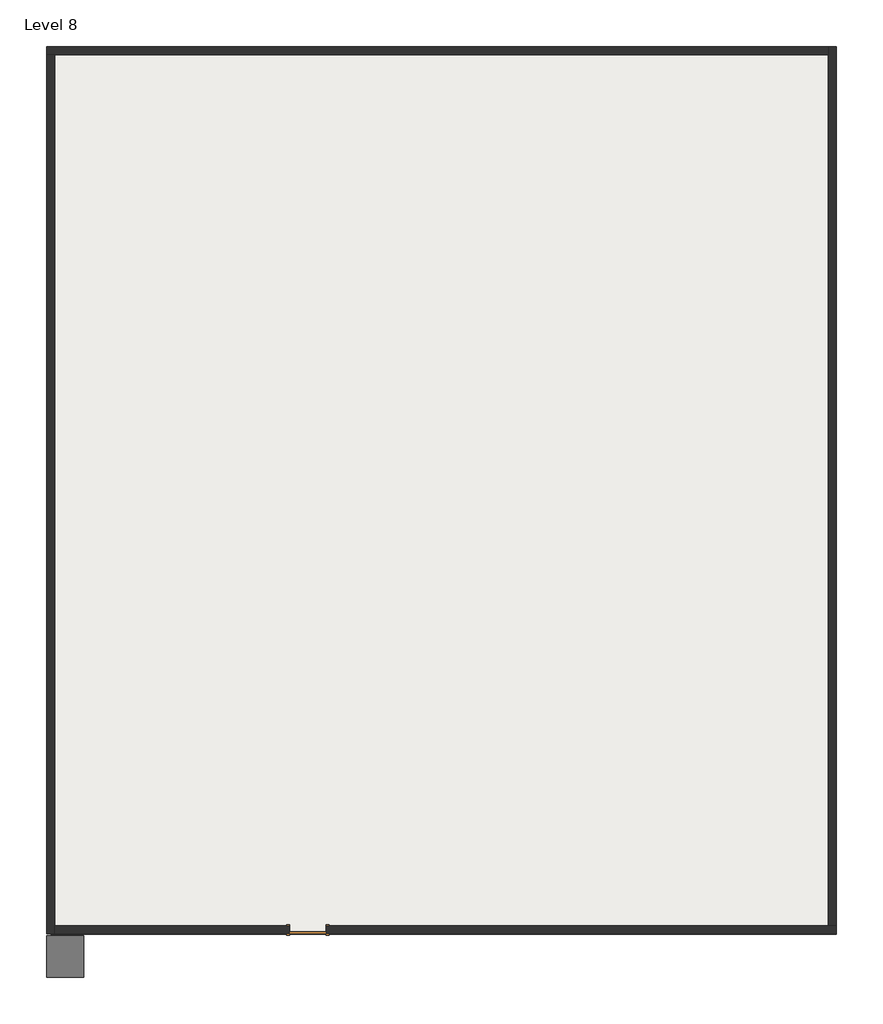
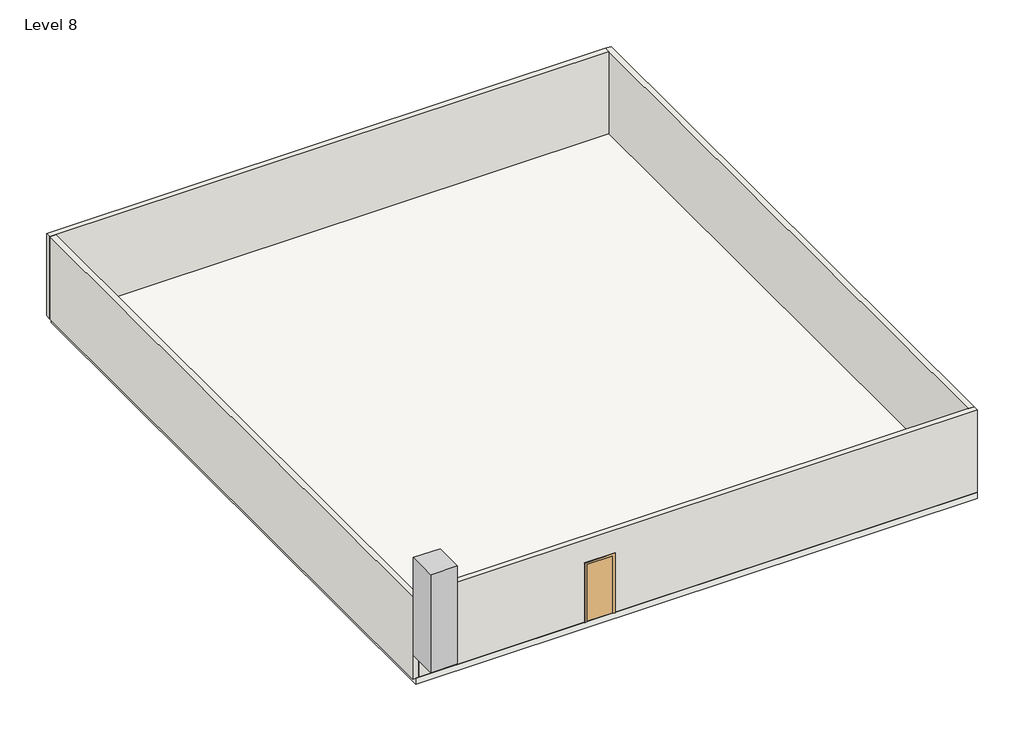
# One storey: 4 walls, 1 door, 1 proxy, 1 roof.
"""IFC4 building model written with IfcOpenShell, lengths in millimetres."""

from ifc_helpers import new_model, si_unit, frame, origin, place, context, project, spatial, polyline, outline, extrude, faceted_brep, transform, mapped, element, save
from components import generic_models_4_generic_models_4_47707f26, door_54dd4da4

model = new_model("IFC4")

# Units and contexts
model_context = context("Model", 3, world=origin())
ifc_project = project(units=[si_unit("LENGTHUNIT", "METRE", prefix="MILLI")], contexts=[model_context])

# Site, building, storey
site = spatial("IfcSite", under=ifc_project)
building = spatial("IfcBuilding", under=site)
storey = spatial("IfcBuildingStorey", under=building, Name="Level 8", Elevation=6553.2)

# Proxy
placement = place(None, origin())
generic_models_4_generic_models_4_shape = generic_models_4_generic_models_4_47707f26(model_context)
element("IfcBuildingElementProxy", 1, Name="Generic Models 4 : Generic Models 4", ObjectType="Generic Models 4 : Generic Models 4", at=placement, inside=storey, context=model_context, shape_type="MappedRepresentation", body=[
    mapped(generic_models_4_generic_models_4_shape, transform((0.0, 0.0, 0.0), x_axis=(1.0, 0.0, 0.0), y_axis=(0.0, 1.0, 0.0), z_axis=(0.0, 0.0, 1.0))),
])

# Door
door_shape = door_54dd4da4(model_context)
element("IfcDoor", 2, ObjectType="Single-Flush : 36\" x 84\"", at=placement, inside=storey, context=model_context, shape_type="MappedRepresentation", body=[
    mapped(door_shape, transform((-3507.5625896, -8539.5821053, 6553.2), x_axis=(-1.0, 0.0, 0.0), y_axis=(0.0, -1.0, 0.0), z_axis=(0.0, 0.0, 1.0))),
])

# Roof
element("IfcRoof", 3, ObjectType="Generic - 9\"", at=placement, inside=storey, context=model_context, shape_type="SweptSolid", body=[
    extrude(outline(polyline([(-9959.1625896, 13507.6178947), (9751.2374104, 13507.6178947), (9751.2374104, -8641.1821053), (-9959.1625896, -8641.1821053), (-9959.1625896, 13507.6178947)])), frame((0.0, 0.0, 6324.6), z_axis=(0.0, 0.0, 1.0), x_axis=(1.0, 0.0, 0.0)), (0.0, 0.0, 1.0), 228.6),
])

# Walls
element("IfcWall", 4, ObjectType="Generic - 8\"", at=placement, inside=storey, context=model_context, shape_type="Brep", body=[
    faceted_brep([(-10060.7625896, 13406.0178947, 6553.2), (-9857.5625896, 13406.0178947, 6553.2), (9548.0374104, 13406.0178947, 6553.2), (9548.0374104, 13406.0178947, 9601.2), (-9857.5625896, 13406.0178947, 9601.2), (-10060.7625896, 13406.0178947, 9601.2), (-10060.7625896, 13609.2178947, 6553.2), (-10060.7625896, 13609.2178947, 9601.2), (9548.0374104, 13609.2178947, 9601.2), (9548.0374104, 13609.2178947, 6553.2)], [[[0, 1, 2, 3, 4, 5]], [[6, 7, 8, 9]], [[2, 1, 0, 6, 9]], [[0, 5, 7, 6]], [[3, 2, 9, 8]], [[5, 4, 3, 8, 7]]]),
])
element("IfcWall", 5, ObjectType="Generic - 8\"", at=placement, inside=storey, context=model_context, shape_type="Brep", body=[
    faceted_brep([(-9857.5625896, -8641.1821053, 6553.2), (-9857.5625896, -8437.9821053, 6553.2), (-9857.5625896, 13406.0178947, 6553.2), (-9857.5625896, 13406.0178947, 9601.2), (-9857.5625896, -8437.9821053, 9601.2), (-9857.5625896, -8641.1821053, 9601.2), (-10060.7625896, -8641.1821053, 6553.2), (-10060.7625896, -8641.1821053, 9601.2), (-10060.7625896, 13406.0178947, 9601.2), (-10060.7625896, 13406.0178947, 6553.2)], [[[0, 1, 2, 3, 4, 5]], [[6, 7, 8, 9]], [[2, 1, 0, 6, 9]], [[0, 5, 7, 6]], [[3, 2, 9, 8]], [[5, 4, 3, 8, 7]]]),
])
element("IfcWall", 6, ObjectType="Generic - 8\"", at=placement, inside=storey, context=model_context, shape_type="Brep", body=[
    faceted_brep([(-3964.7625896, -8437.9821053, 8686.8), (-3964.7625896, -8437.9821053, 6553.2), (-9857.5625896, -8437.9821053, 6553.2), (-9857.5625896, -8437.9821053, 9601.2), (9548.0374104, -8437.9821053, 9601.2), (9751.2374104, -8437.9821053, 9601.2), (9751.2374104, -8437.9821053, 6553.2), (9548.0374104, -8437.9821053, 6553.2), (-3050.3625896, -8437.9821053, 6553.2), (-3050.3625896, -8437.9821053, 8686.8), (-9857.5625896, -8641.1821053, 6553.2), (-3964.7625896, -8641.1821053, 6553.2), (-3964.7625896, -8641.1821053, 8686.8), (-3050.3625896, -8641.1821053, 8686.8), (-3050.3625896, -8641.1821053, 6553.2), (9751.2374104, -8641.1821053, 6553.2), (9751.2374104, -8641.1821053, 9601.2), (-9857.5625896, -8641.1821053, 9601.2)], [[[0, 1, 2, 3, 4, 5, 6, 7, 8, 9]], [[10, 11, 12, 13, 14, 15, 16, 17]], [[2, 1, 11, 10]], [[8, 7, 6, 15, 14]], [[6, 5, 16, 15]], [[3, 2, 10, 17]], [[5, 4, 3, 17, 16]], [[12, 11, 1, 0]], [[13, 12, 0, 9]], [[14, 13, 9, 8]]]),
])
element("IfcWall", 7, ObjectType="Generic - 8\"", at=placement, inside=storey, context=model_context, shape_type="Brep", body=[
    faceted_brep([(9548.0374104, 13609.2178947, 6553.2), (9548.0374104, 13406.0178947, 6553.2), (9548.0374104, -8437.9821053, 6553.2), (9548.0374104, -8437.9821053, 9601.2), (9548.0374104, 13406.0178947, 9601.2), (9548.0374104, 13609.2178947, 9601.2), (9751.2374104, 13609.2178947, 6553.2), (9751.2374104, 13609.2178947, 9601.2), (9751.2374104, -8437.9821053, 9601.2), (9751.2374104, -8437.9821053, 6553.2)], [[[0, 1, 2, 3, 4, 5]], [[6, 7, 8, 9]], [[2, 1, 0, 6, 9]], [[0, 5, 7, 6]], [[3, 2, 9, 8]], [[5, 4, 3, 8, 7]]]),
])

save(model, "model.ifc")

# Revit data of these elements
# Type "Single-Flush : 36\" x 84\""
#   Type Mark = "1"
#   Construction Type Id = "MDOOR"
#   Assembly Code = "C1020"
#   Analytic Construction = "Metal"
#   Thickness = 0' - 2"
#   Heat Transfer Coefficient (U) = 0.651978 BTU/(h·ft²·°F)
#   Height = 7' - 0"
#   Trim Projection Ext = 0' - 1"
#   Trim Projection Int = 0' - 1"
#   Trim Width = 0' - 3"
#   Width = 3' - 0"
#   Define Thermal Properties by = 1
#   Door Material = Door - Panel
#   Frame Material = Door - Frame
#   Visual Light Transmittance = 0
#   Solar Heat Gain Coefficient = 0
#   Function = (empty or 0)
#   Wall Closure = (empty or 0)
# Type "Generic - 9\""
#   Assembly Code = "B1020"
#   Layers, outside or top first: 0' - 9" no material (function 1)
# Type "Generic - 8\""
#   Assembly Code = "B2010"
#   Layers, outside or top first: 0' - 8" no material (function 1)
# Element 1 (IfcBuildingElementProxy, "Generic Models 4 : Generic Models 4")
#   Phase Created = New Construction
# Element 2 (IfcDoor, "Single-Flush : 36\" x 84\"")
#   Phase Created = New Construction
#   Materials on its faces: "Door - Frame", "Door - Panel"
# Element 3 (IfcRoof, "Generic - 9\"")
#   built-in parameter 1001705 = 21.5 (stored number, unit not read)
#   built-in parameter 1001701 = -0.75 (stored number, unit not read)
#   built-in parameter 1001710 = 33615
#   Phase Created = New Construction
#   Materials on its faces: "Default Roof"
# Elements 4, 5, 6, 7 (IfcWall, "Generic - 8\"")
#   Top Offset = 0' - 0"
#   Base Offset = 0' - 0"
#   Unconnected Height = 10' - 0"
#   wall height = 10' - 0"
#   Phase Created = New Construction
#   Base Constraint = Level 8
#   Materials on its faces: "Default Wall"
# Materials
#   "Door - Panel": class "Wood", colour RGB 210 159 95, transparency 0
#   "Door - Frame": colour RGB 118 70 51, transparency 0
#   "Default Roof": colour RGB 88 101 114, transparency 0
#   "Default Wall": colour RGB 128 128 128, transparency 0
